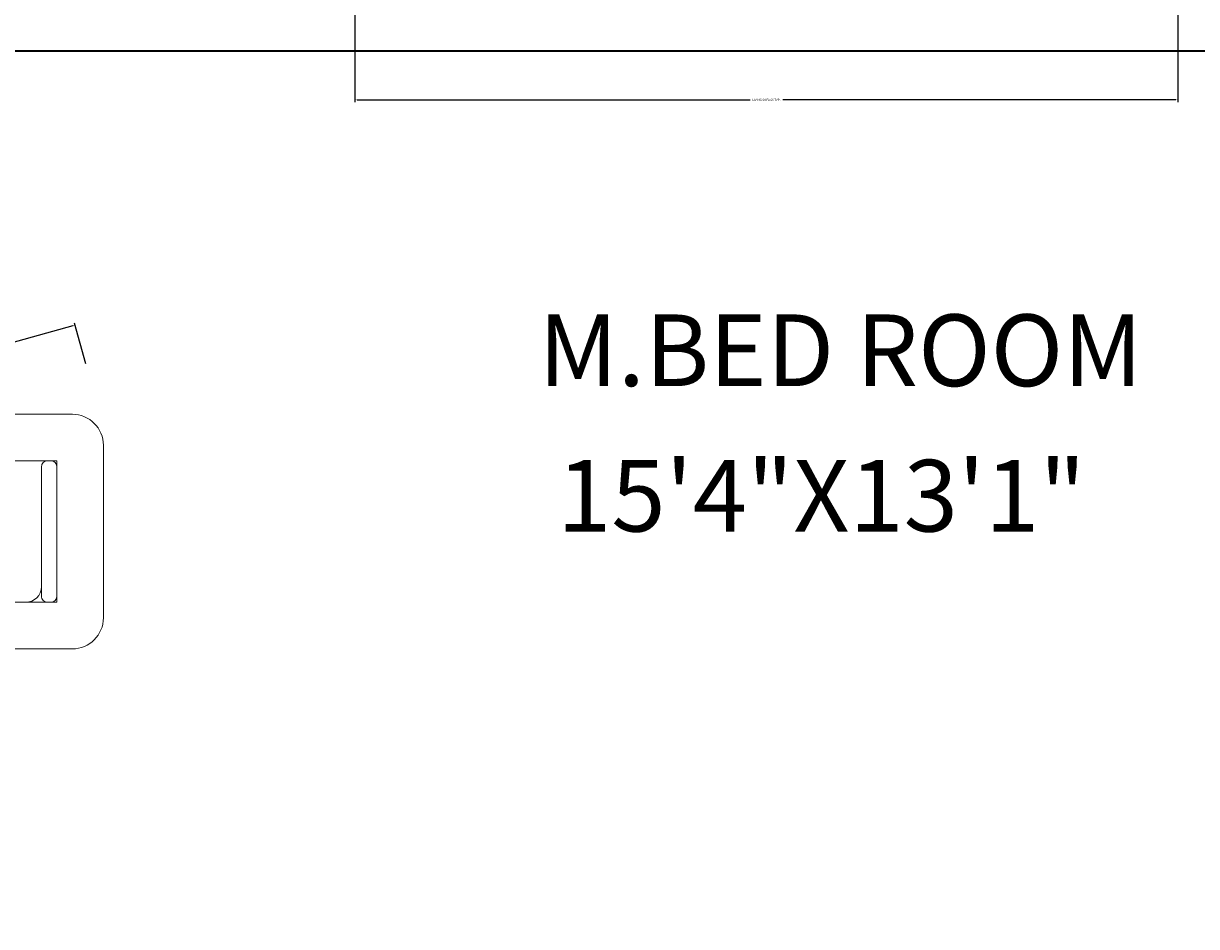
# Model space of a CAD drawing. Units: millimetres. Extents: x 27017497 to 27018854, y 7058029 to 7059154.
# Tile 28 of 91: x 27017651 to 27017748, y 7058222 to 7058297. Entities that reach past the tile are written whole.
import ezdxf

# ---------------------------------------------------------------- set-up
doc = ezdxf.new("R2010")
doc.units = ezdxf.units.MM
for name, color, linetype, lineweight in [('A-ANNO-DIMS', 2, 'Continuous', 18), ('A-AREA-IDEN', 7, 'Continuous', 18), ('A-FURN', 8, 'Continuous', 18), ('A-WALL', 7, 'Continuous', 35)]:
    doc.layers.add(name, color=color, linetype=linetype, lineweight=lineweight)
doc.styles.get("Standard").update_dxf_attribs({"font": 'arial.ttf'})
doc.dimstyles.get("Standard").update_dxf_attribs({"dimtxt": 0.18, "dimasz": 0.18, "dimexe": 0.18, "dimexo": 0.0625, "dimgap": 0.09, "dimtad": 0, "dimtih": 1, "dimtoh": 1, "dimdec": 4, "dimzin": 0, "dimdsep": 46, "dimtxsty": 'Standard', "dimcen": 0.09, "dimadec": 0, "dimazin": 0, "dimtfac": 1, "dimtdec": 4, "dimtofl": 0, "dimtmove": 0, "dimatfit": 3, "dimfxl": 1, "dimtolj": 1, "dimtzin": 0, "dimarcsym": 0})

# ---------------------------------------------------------------- blocks, each defined once
blk = doc.blocks.new('CHAIR-OCCASIONAL')
for p, q in [((19.599, 18.742), (7.02, 22.21)), ((3.873, 20.423), (0.092, 6.706)), ((4.132, 6.919), (7.234, 18.169)), ((5.25, 10.974), (7.234, 18.169)), ((5.25, 10.974), (7.098, 17.676)), ((16.064, 15.735), (7.234, 18.169)), ((7.234, 18.169), (16.064, 15.735)), ((7.234, 18.169), (16.064, 15.735)), ((7.727, 18.033), (7.974, 17.965)), ((7.727, 18.033), (7.974, 17.965)), ((17.638, 16.628), (17.978, 17.862)), ((17.638, 16.628), (17.978, 17.862)), ((8.331, 17.336), (5.625, 7.52)), ((17.605, 1.878), (21.386, 15.595)), ((12.963, 4.485), (4.132, 6.919)), ((4.872, 6.715), (4.626, 6.783)), ((5.625, 7.52), (5.502, 7.072)), ((1.879, 3.558), (14.458, 0.091)), ((13.856, 2.911), (13.516, 1.678))]:
    blk.add_line(p, q)
for centre, radius, start, end in [((6.34, 19.743), 2.559, 74.58786, 164.58786), ((16.744, 18.202), 1.28, 344.58786, 74.58786), ((16.744, 18.202), 1.28, 344.58786, 74.58786), ((18.919, 16.275), 2.559, 344.58786, 74.58786), ((7.591, 17.54), 0.512, 74.58786, 164.58786), ((7.838, 17.472), 0.512, 344.58786, 74.58786), ((9.361, 16.256), 1.28, 74.58786, 164.58786), ((16.404, 16.968), 1.28, 254.58786, 344.58786), ((16.404, 16.968), 1.28, 254.58786, 344.58786), ((4.762, 7.276), 0.512, 164.58786, 254.58786), ((5.008, 7.208), 0.512, 254.58786, 344.58786), ((2.559, 6.025), 2.559, 164.58786, 254.58786), ((12.623, 3.251), 1.28, 344.58786, 74.58786), ((12.283, 2.018), 1.28, 254.58786, 344.58786), ((15.138, 2.558), 2.559, 254.58786, 344.58786)]:
    blk.add_arc(centre, radius, start, end)
blk = doc.blocks.new('*D22')
at = {"layer": 'A-ANNO-DIMS', "color": 0, "lineweight": -2, "transparency": 16777216}
for p, q in [((27017656.18, 7058268.579), (27017655.252, 7058271.943)), ((27017655.127, 7058271.722), (27017645.203, 7058268.986)), ((27017634.221, 7058265.959), (27017644.144, 7058268.694)), ((27017634.927, 7058262.72), (27017633.999, 7058266.084))]:
    blk.add_line(p, q, dxfattribs=at)
at = {"layer": 'A-ANNO-DIMS', "color": 0, "transparency": 16777216}
for points in [[(27017655.119, 7058271.751), (27017655.135, 7058271.693), (27017655.3, 7058271.77)], [(27017634.213, 7058265.987), (27017634.229, 7058265.93), (27017634.047, 7058265.911)]]:
    blk.add_solid(points, dxfattribs=at)
at = {"layer": 'Defpoints', "color": 0, "transparency": 16777216}
for p in [(27017656.196, 7058268.519), (27017634.047, 7058265.911), (27017634.943, 7058262.66)]:
    blk.add_point(p, dxfattribs=at)
at = {"layer": 'A-ANNO-DIMS', "color": 0, "transparency": 16777216, "insert": (27017644.674, 7058268.84), "char_height": 0.18, "attachment_point": 5}
blk.add_mtext('\\A1;22 TYP.', dxfattribs=at)
blk = doc.blocks.new('*D39')
at = {"layer": 'A-ANNO-DIMS', "color": 0, "lineweight": -2, "transparency": 16777216}
for p, q in [((27017678.38, 7058300.482), (27017678.38, 7058290.182)), ((27017746.263, 7058300.482), (27017746.263, 7058290.182)), ((27017678.56, 7058290.362), (27017710.973, 7058290.362)), ((27017746.083, 7058290.362), (27017713.67, 7058290.362))]:
    blk.add_line(p, q, dxfattribs=at)
at = {"layer": 'A-ANNO-DIMS', "color": 0, "transparency": 16777216}
for points in [[(27017678.56, 7058290.392), (27017678.56, 7058290.332), (27017678.38, 7058290.362)], [(27017746.083, 7058290.392), (27017746.083, 7058290.332), (27017746.263, 7058290.362)]]:
    blk.add_solid(points, dxfattribs=at)
at = {"layer": 'Defpoints', "color": 0, "transparency": 16777216}
for p in [(27017678.38, 7058300.544), (27017746.263, 7058300.544), (27017746.263, 7058290.362)]:
    blk.add_point(p, dxfattribs=at)
at = {"layer": 'A-ANNO-DIMS', "color": 0, "transparency": 16777216, "insert": (27017712.321, 7058290.362), "char_height": 0.18, "attachment_point": 5}
blk.add_mtext('\\A1;LIVING SOFA 68 TYP.', dxfattribs=at)
blk = doc.blocks.new('*D47')
at = {"layer": 'A-ANNO-DIMS', "color": 0, "lineweight": -2, "transparency": 16777216}
for p, q in [((27017561.166, 7058294.35), (27017561.166, 7058028.6)), ((27018790.606, 7058294.35), (27018790.606, 7058028.6)), ((27017561.346, 7058028.78), (27018175.431, 7058028.78)), ((27018790.426, 7058028.78), (27018176.341, 7058028.78))]:
    blk.add_line(p, q, dxfattribs=at)
at = {"layer": 'A-ANNO-DIMS', "color": 0, "transparency": 16777216}
for points in [[(27017561.346, 7058028.81), (27017561.346, 7058028.75), (27017561.166, 7058028.78)], [(27018790.426, 7058028.81), (27018790.426, 7058028.75), (27018790.606, 7058028.78)]]:
    blk.add_solid(points, dxfattribs=at)
at = {"layer": 'Defpoints', "color": 0, "transparency": 16777216}
for p in [(27017561.166, 7058294.412), (27018790.606, 7058294.412), (27018790.606, 7058028.78)]:
    blk.add_point(p, dxfattribs=at)
at = {"layer": 'A-ANNO-DIMS', "color": 0, "transparency": 16777216, "insert": (27018175.886, 7058028.78), "char_height": 0.18, "attachment_point": 5}
blk.add_mtext('\\A1;1229.4', dxfattribs=at)
blk = doc.blocks.new('*D48')
at = {"layer": 'A-ANNO-DIMS', "color": 0, "lineweight": -2, "transparency": 16777216}
for p, q in [((27018463.498, 7058622.912), (27017497.536, 7058622.912)), ((27017497.716, 7058622.732), (27017497.716, 7058357.753)), ((27017497.716, 7058092.41), (27017497.716, 7058357.389)), ((27018555.129, 7058092.23), (27017497.536, 7058092.23))]:
    blk.add_line(p, q, dxfattribs=at)
at = {"layer": 'A-ANNO-DIMS', "color": 0, "transparency": 16777216}
for points in [[(27017497.686, 7058622.732), (27017497.746, 7058622.732), (27017497.716, 7058622.912)], [(27017497.686, 7058092.41), (27017497.746, 7058092.41), (27017497.716, 7058092.23)]]:
    blk.add_solid(points, dxfattribs=at)
at = {"layer": 'Defpoints', "color": 0, "transparency": 16777216}
for p in [(27018463.561, 7058622.912), (27017497.716, 7058092.23), (27018555.192, 7058092.23)]:
    blk.add_point(p, dxfattribs=at)
at = {"layer": 'A-ANNO-DIMS', "color": 0, "transparency": 16777216, "insert": (27017497.716, 7058357.571), "char_height": 0.18, "attachment_point": 5}
blk.add_mtext('\\A1;530.7', dxfattribs=at)

msp = doc.modelspace()

# ---------------------------------------------------------------- linework, layer by layer
at = {"layer": 'A-WALL'}
msp.add_line((27017622.666, 7058294.412), (27017758.765, 7058294.412), dxfattribs=at)

# ---------------------------------------------------------------- block references
at = {"layer": 'A-FURN', "rotation": 195.4121391531662}
msp.add_blockref('CHAIR-OCCASIONAL', (27017655.946, 7058268.357), dxfattribs=at)

# ---------------------------------------------------------------- texts
at = {"layer": 'A-ANNO-DIMS'}
msp.add_text('15\'4"X13\'1"', height=5.91176, dxfattribs=at).set_placement((27017695.053, 7058254.754))
at = {"layer": 'A-AREA-IDEN'}
msp.add_text('M.BED ROOM', height=5.9118, dxfattribs=at).set_placement((27017693.518, 7058266.751))

# ---------------------------------------------------------------- dimensions: what is measured, and where the dimension line sits
at = {"layer": 'A-ANNO-DIMS'}
dim = msp.add_linear_dim(base=(27017497.716, 7058092.23), p1=(27018463.561, 7058622.912), p2=(27018555.192, 7058092.23), angle=90, dimstyle='Standard', override={"dimdec": 1, "dimlfac": 1, "dimrnd": 0, "dimzin": 0, "dimdsep": 46, "dimlunit": 2}, dxfattribs=at)
dim.commit()
dim.dimension.update_dxf_attribs({"geometry": '*D48', "text_midpoint": (27017497.716, 7058357.571)})
dim = msp.add_linear_dim(base=(27017746.263, 7058290.362), p1=(27017678.38, 7058300.544), p2=(27017746.263, 7058300.544), text='LIVING SOFA <> TYP.', dimstyle='Standard', override={"dimdec": 0, "dimlfac": 1, "dimrnd": 0, "dimzin": 0, "dimdsep": 46, "dimlunit": 2}, dxfattribs=at)
dim.commit()
dim.dimension.update_dxf_attribs({"geometry": '*D39', "text_midpoint": (27017712.321, 7058290.362)})
dim = msp.add_linear_dim(base=(27018790.606, 7058028.78), p1=(27017561.166, 7058294.412), p2=(27018790.606, 7058294.412), dimstyle='Standard', override={"dimdec": 1, "dimlfac": 1, "dimrnd": 0, "dimzin": 0, "dimdsep": 46, "dimlunit": 2}, dxfattribs=at)
dim.commit()
dim.dimension.update_dxf_attribs({"geometry": '*D47', "text_midpoint": (27018175.886, 7058028.78)})
dim = msp.add_linear_dim(base=(27017634.047, 7058265.911), p1=(27017656.196, 7058268.519), p2=(27017634.943, 7058262.66), angle=195.41214, text='<> TYP.', dimstyle='Standard', override={"dimdec": 0, "dimlfac": 1, "dimrnd": 0, "dimzin": 0, "dimdsep": 46, "dimlunit": 2}, dxfattribs=at)
dim.commit()
dim.dimension.update_dxf_attribs({"geometry": '*D22', "text_midpoint": (27017644.674, 7058268.84)})

doc.saveas('drawing.dxf')
